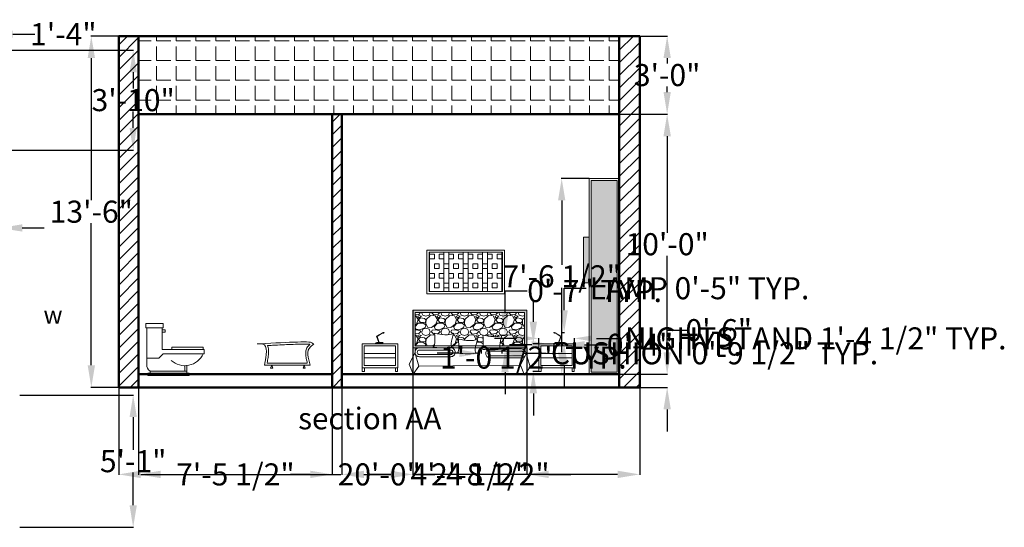
# Model space of a CAD drawing. Units: inches. Extents: x 4451 to 5261, y 886 to 1442.
# Tile 3 of 4: x 4807 to 5261, y 928 to 1162. Entities that reach past the tile are written whole.
import ezdxf

# ---------------------------------------------------------------- set-up
doc = ezdxf.new("R2010")
doc.units = ezdxf.units.IN
doc.header["$MEASUREMENT"] = 0
for name, color, linetype, lineweight in [('A-ANNO-DIMS', 2, 'Continuous', 18), ('A-ANNO-TEXT', 7, 'Continuous', 25), ('A-FLOR-FIXT', 9, 'Continuous', 20), ('A-FURN', 8, 'Continuous', 18), ('A-FURN-PATT', 8, 'Continuous', 13), ('A-SECT', 7, 'Continuous', 50)]:
    doc.layers.add(name, color=color, linetype=linetype, lineweight=lineweight)
doc.layers.add('A-SECT-PATT', color=241, linetype='Continuous', lineweight=13, true_color=0xf7abae)
doc.styles.get("Standard").update_dxf_attribs({"font": 'arial.ttf'})
doc.dimstyles.get("Standard").update_dxf_attribs({"dimtxt": 10.18, "dimasz": 10.18, "dimexe": 0.18, "dimexo": 0.0625, "dimgap": 0.09, "dimtad": 0, "dimtih": 1, "dimtoh": 1, "dimdec": 0, "dimzin": 0, "dimdsep": 46, "dimlunit": 3, "dimtxsty": 'Standard', "dimcen": 0.09, "dimadec": 0, "dimazin": 0, "dimtfac": 1, "dimtdec": 0, "dimtofl": 0, "dimtmove": 0, "dimatfit": 3, "dimfxl": 1, "dimtolj": 1, "dimtzin": 0, "dimarcsym": 0})
pattern_1 = [(45, (-229.911, 0), (-2.9168155, 2.9168155), [])]

# ---------------------------------------------------------------- blocks, each defined once
blk = doc.blocks.new('*U10')
for p, q in [((-0.5, 5), (-0.5, 22)), ((6.5, 22), (6.5, 12)), ((6.5, 21), (8, 21)), ((8, 20), (6.5, 20)), ((8, 21), (8, 20)), ((7, 10), (5, 8)), ((6.5, 12), (26, 12)), ((26, 10), (7, 10)), ((11, 13), (11, 12)), ((25.5, 13), (11, 13)), ((25.5, 12), (25.5, 13)), ((26, 12), (26, 10)), ((5, 8), (-0.5, 8)), ((1, 2), (1, 1)), ((18, 2), (1, 2)), ((17, 4.5), (17, 2)), ((18, 2), (18, 4.5376)), ((18, 1), (18, 2))]:
    blk.add_line(p, q)
for points in [[(-1, 22), (-1, 24), (7, 24), (7, 22)], [(0, 0), (0, 1), (19, 1), (19, 0)]]:
    blk.add_lwpolyline(points, close=True)
for centre, radius, start, end in [((17, 13.7955), 9.3089, 227.7453, 335.9381), ((2.75, 4.75), 3.2596, 175.6013, 237.5288)]:
    blk.add_arc(centre, radius, start, end)
blk = doc.blocks.new('CUSHION-ELEV')
for points in [[(0.79, 6.75), (0.98, 3.53), (1.17, 0.31), (0, 0.27)], [(0.79, 6.75), (4.1, 6.13), (7.4, 5.52), (9.55, 6.75)], [(0, 0.27), (2.47, 0.04), (4.94, -0.18), (9.29, 0.22)]]:
    blk.add_open_spline(points, degree=3)
blk.add_open_spline([(9.55, 6.75), (8.66, 3.34), (7.77, -0.07), (9.51, 0.25), (9.51, 0.25)], degree=3, knots=[0, 0, 0, 0, 6.500705, 6.513641, 6.513641, 6.513641, 6.513641])
blk = doc.blocks.new('NIGHTSTAND-ELEV')
for p, q in [((1, 8.22), (15.46, 8.22)), ((1, 8.22), (15.46, 8.22)), ((1, 6.22), (15.46, 6.22))]:
    blk.add_line(p, q)
for points in [[(0, 12.74), (0, 12.74), (16.46, 12.74), (16.46, 12.74), (16.46, 1.69), (16.46, 1.69), (0, 1.69), (0, 1.69)], [(1, 11.74), (15.46, 11.74), (15.46, 2.69), (1, 2.69)], [(1.07, 1.69), (1.07, 1.69), (0.06, 1.69), (0.06, 1.69), (0.06, 0), (0.06, 0), (1.07, 0), (1.07, 0)], [(16.41, 1.69), (16.41, 1.69), (15.4, 1.69), (15.4, 1.69), (15.4, 0), (15.4, 0), (16.41, 0), (16.41, 0)]]:
    blk.add_lwpolyline(points, close=True)
blk = doc.blocks.new('BEDSIDE-LAMP-ELEV')
for p, q in [((0.39, 4.98), (0, 4.98)), ((3.41, 3.22), (0.39, 4.98)), ((3.22, 3.15), (0.65, 4.7)), ((0.75, 0.34), (0.36, 0)), ((0.36, 0), (4.03, 0)), ((3.35, 0.34), (0.75, 0.34)), ((2.21, 0.34), (3.22, 3.15)), ((2.36, 0.34), (3.41, 3.22)), ((4.03, 0), (3.35, 0.34))]:
    blk.add_line(p, q)
blk.add_arc((0.39, 4.98), 0.387, 180, 329.7191)
blk = doc.blocks.new('*D30')
at = {"layer": 'A-ANNO-DIMS', "color": 0, "lineweight": -2, "transparency": 16777216}
for p, q in [((4777.87, 1159.67), (4777.87, 1155.48)), ((4793.72, 1159.67), (4793.72, 1155.48)), ((4767.69, 1155.66), (4757.51, 1155.66)), ((4803.9, 1155.66), (4814.08, 1155.66))]:
    blk.add_line(p, q, dxfattribs=at)
at = {"layer": 'A-ANNO-DIMS', "color": 0, "transparency": 16777216}
for points in [[(4767.69, 1157.36), (4767.69, 1153.97), (4777.87, 1155.66)], [(4803.9, 1157.36), (4803.9, 1153.97), (4793.72, 1155.66)]]:
    blk.add_solid(points, dxfattribs=at)
at = {"layer": 'Defpoints', "color": 0, "transparency": 16777216}
for p in [(4777.87, 1159.74), (4793.72, 1159.74), (4793.72, 1155.66)]:
    blk.add_point(p, dxfattribs=at)
at = {"layer": 'A-ANNO-DIMS', "color": 0, "transparency": 16777216, "insert": (4827.22, 1155.66), "char_height": 10.18, "attachment_point": 5}
blk.add_mtext('\\A1;1\'-4"', dxfattribs=at)
blk = doc.blocks.new('*D35')
at = {"layer": 'A-ANNO-DIMS', "color": 0, "lineweight": -2, "transparency": 16777216}
for p, q in [((5009.76, 1008.51), (4999.58, 1008.51)), ((5019.94, 1009.88), (5019.94, 1008.33)), ((5029.48, 1009.88), (5029.48, 1008.33)), ((5039.66, 1008.51), (5049.84, 1008.51))]:
    blk.add_line(p, q, dxfattribs=at)
at = {"layer": 'A-ANNO-DIMS', "color": 0, "transparency": 16777216}
for points in [[(5009.76, 1010.2), (5009.76, 1006.81), (5019.94, 1008.51)], [(5039.66, 1010.2), (5039.66, 1006.81), (5029.48, 1008.51)]]:
    blk.add_solid(points, dxfattribs=at)
at = {"layer": 'Defpoints', "color": 0, "transparency": 16777216}
for p in [(5019.94, 1009.94), (5029.48, 1009.94), (5029.48, 1008.51)]:
    blk.add_point(p, dxfattribs=at)
at = {"layer": 'A-ANNO-DIMS', "color": 0, "transparency": 16777216, "insert": (5127.53, 1008.51), "char_height": 10.18, "attachment_point": 5}
blk.add_mtext('\\A1;CUSHION 0\'-9 1/2" TYP.', dxfattribs=at)
blk = doc.blocks.new('*D36')
at = {"layer": 'A-ANNO-DIMS', "color": 0, "lineweight": -2, "transparency": 16777216}
for p, q in [((5030.92, 1027.05), (5030.92, 1037.23)), ((5030.92, 1037.23), (5041.1, 1037.23)), ((5029.55, 1016.87), (5031.1, 1016.87)), ((5029.55, 1009.94), (5031.1, 1009.94)), ((5030.92, 999.76), (5030.92, 989.58))]:
    blk.add_line(p, q, dxfattribs=at)
at = {"layer": 'A-ANNO-DIMS', "color": 0, "transparency": 16777216}
for points in [[(5029.22, 1027.05), (5032.61, 1027.05), (5030.92, 1016.87)], [(5029.22, 999.76), (5032.61, 999.76), (5030.92, 1009.94)]]:
    blk.add_solid(points, dxfattribs=at)
at = {"layer": 'Defpoints', "color": 0, "transparency": 16777216}
for p in [(5029.48, 1016.87), (5030.92, 1016.87), (5029.48, 1009.94)]:
    blk.add_point(p, dxfattribs=at)
at = {"layer": 'A-ANNO-DIMS', "color": 0, "transparency": 16777216, "insert": (5072.21, 1037.23), "char_height": 10.18, "attachment_point": 5}
blk.add_mtext('\\A1;0\'-7" TYP.', dxfattribs=at)
blk = doc.blocks.new('*D37')
at = {"layer": 'A-ANNO-DIMS', "color": 0, "lineweight": -2, "transparency": 16777216}
for p, q in [((5058.17, 1028.33), (5058.17, 1038.51)), ((5058.17, 1038.51), (5068.35, 1038.51)), ((5057.48, 1018.15), (5058.35, 1018.15)), ((5057.48, 1013.17), (5058.35, 1013.17)), ((5058.17, 1002.99), (5058.17, 992.81))]:
    blk.add_line(p, q, dxfattribs=at)
at = {"layer": 'A-ANNO-DIMS', "color": 0, "transparency": 16777216}
for points in [[(5056.47, 1028.33), (5059.86, 1028.33), (5058.17, 1018.15)], [(5056.47, 1002.99), (5059.86, 1002.99), (5058.17, 1013.17)]]:
    blk.add_solid(points, dxfattribs=at)
at = {"layer": 'Defpoints', "color": 0, "transparency": 16777216}
for p in [(5057.42, 1018.15), (5058.17, 1018.15), (5057.42, 1013.17)]:
    blk.add_point(p, dxfattribs=at)
at = {"layer": 'A-ANNO-DIMS', "color": 0, "transparency": 16777216, "insert": (5120.58, 1038.51), "char_height": 10.18, "attachment_point": 5}
blk.add_mtext('\\A1;LAMP 0\'-5" TYP.', dxfattribs=at)
blk = doc.blocks.new('*D38')
at = {"layer": 'A-ANNO-DIMS', "color": 0, "lineweight": -2, "transparency": 16777216}
for p, q in [((5053.39, 1013.1), (5053.39, 1012.24)), ((5057.42, 1013.1), (5057.42, 1012.24)), ((5043.21, 1012.42), (5033.03, 1012.42)), ((5067.6, 1012.42), (5077.78, 1012.42))]:
    blk.add_line(p, q, dxfattribs=at)
at = {"layer": 'A-ANNO-DIMS', "color": 0, "transparency": 16777216}
for points in [[(5043.21, 1014.12), (5043.21, 1010.72), (5053.39, 1012.42)], [(5067.6, 1014.12), (5067.6, 1010.72), (5057.42, 1012.42)]]:
    blk.add_solid(points, dxfattribs=at)
at = {"layer": 'Defpoints', "color": 0, "transparency": 16777216}
for p in [(5053.39, 1013.17), (5057.42, 1013.17), (5057.42, 1012.42)]:
    blk.add_point(p, dxfattribs=at)
at = {"layer": 'A-ANNO-DIMS', "color": 0, "transparency": 16777216, "insert": (5108.9, 1012.42), "char_height": 10.18, "attachment_point": 5}
blk.add_mtext('\\A1;0\'-4" TYP.', dxfattribs=at)
blk = doc.blocks.new('*D39')
at = {"layer": 'A-ANNO-DIMS', "color": 0, "lineweight": -2, "transparency": 16777216}
for p, q in [((5036.25, 1015.37), (5026.07, 1015.37)), ((5046.43, 1012.96), (5046.43, 1015.55)), ((5062.9, 1012.96), (5062.9, 1015.55)), ((5073.08, 1015.37), (5083.26, 1015.37))]:
    blk.add_line(p, q, dxfattribs=at)
at = {"layer": 'A-ANNO-DIMS', "color": 0, "transparency": 16777216}
for points in [[(5036.25, 1017.06), (5036.25, 1013.67), (5046.43, 1015.37)], [(5073.08, 1017.06), (5073.08, 1013.67), (5062.9, 1015.37)]]:
    blk.add_solid(points, dxfattribs=at)
at = {"layer": 'Defpoints', "color": 0, "transparency": 16777216}
for p in [(5046.43, 1012.9), (5062.9, 1015.37), (5062.9, 1012.9)]:
    blk.add_point(p, dxfattribs=at)
at = {"layer": 'A-ANNO-DIMS', "color": 0, "transparency": 16777216, "insert": (5174.18, 1015.37), "char_height": 10.18, "attachment_point": 5}
blk.add_mtext('\\A1;NIGHTSTAND 1\'-4 1/2" TYP.', dxfattribs=at)
blk = doc.blocks.new('*D40')
at = {"layer": 'A-ANNO-DIMS', "color": 0, "lineweight": -2, "transparency": 16777216}
for p, q in [((5043.96, 1023.08), (5043.96, 1033.26)), ((5046.37, 1012.9), (5043.78, 1012.9)), ((5046.37, 1000.16), (5043.78, 1000.16)), ((5043.96, 989.98), (5043.96, 979.8))]:
    blk.add_line(p, q, dxfattribs=at)
at = {"layer": 'A-ANNO-DIMS', "color": 0, "transparency": 16777216}
for points in [[(5042.27, 1023.08), (5045.66, 1023.08), (5043.96, 1012.9)], [(5042.27, 989.98), (5045.66, 989.98), (5043.96, 1000.16)]]:
    blk.add_solid(points, dxfattribs=at)
at = {"layer": 'Defpoints', "color": 0, "transparency": 16777216}
for p in [(5043.96, 1012.9), (5046.43, 1012.9), (5046.43, 1000.16)]:
    blk.add_point(p, dxfattribs=at)
at = {"layer": 'A-ANNO-DIMS', "color": 0, "transparency": 16777216, "insert": (5043.96, 1006.53), "char_height": 10.18, "attachment_point": 5}
blk.add_mtext('\\A1;1\'-0 1/2" TYP.', dxfattribs=at)
blk = doc.blocks.new('*D44')
at = {"layer": 'A-ANNO-DIMS', "color": 0, "lineweight": -2, "transparency": 16777216}
for p, q in [((4807.16, 989.25), (4859.61, 989.25)), ((4859.43, 979.07), (4859.43, 964.04)), ((4859.43, 938.43), (4859.43, 953.46)), ((4807.16, 928.25), (4859.61, 928.25))]:
    blk.add_line(p, q, dxfattribs=at)
at = {"layer": 'A-ANNO-DIMS', "color": 0, "transparency": 16777216}
for points in [[(4857.74, 979.07), (4861.13, 979.07), (4859.43, 989.25)], [(4857.74, 938.43), (4861.13, 938.43), (4859.43, 928.25)]]:
    blk.add_solid(points, dxfattribs=at)
at = {"layer": 'Defpoints', "color": 0, "transparency": 16777216}
for p in [(4807.09, 989.25), (4859.43, 989.25), (4807.09, 928.25)]:
    blk.add_point(p, dxfattribs=at)
at = {"layer": 'A-ANNO-DIMS', "color": 0, "transparency": 16777216, "insert": (4859.43, 958.75), "char_height": 10.18, "attachment_point": 5}
blk.add_mtext('\\A1;5\'-1"', dxfattribs=at)
blk = doc.blocks.new('*D45')
at = {"layer": 'A-ANNO-DIMS', "color": 0, "lineweight": -2, "transparency": 16777216}
for p, q in [((4798.16, 1148.25), (4859.61, 1148.25)), ((4859.43, 1138.07), (4859.43, 1130.54)), ((4859.43, 1112.43), (4859.43, 1119.96)), ((4798.16, 1102.25), (4859.61, 1102.25))]:
    blk.add_line(p, q, dxfattribs=at)
at = {"layer": 'A-ANNO-DIMS', "color": 0, "transparency": 16777216}
for points in [[(4857.74, 1138.07), (4861.13, 1138.07), (4859.43, 1148.25)], [(4857.74, 1112.43), (4861.13, 1112.43), (4859.43, 1102.25)]]:
    blk.add_solid(points, dxfattribs=at)
at = {"layer": 'Defpoints', "color": 0, "transparency": 16777216}
for p in [(4798.09, 1148.25), (4859.43, 1148.25), (4798.09, 1102.25)]:
    blk.add_point(p, dxfattribs=at)
at = {"layer": 'A-ANNO-DIMS', "color": 0, "transparency": 16777216, "insert": (4859.43, 1125.25), "char_height": 10.18, "attachment_point": 5}
blk.add_mtext('\\A1;3\'-10"', dxfattribs=at)
blk = doc.blocks.new('*D55')
at = {"layer": 'A-ANNO-DIMS', "color": 0, "lineweight": -2, "transparency": 16777216}
for p, q in [((4786.59, 1093.19), (4786.59, 1066.12)), ((4798.09, 1093.19), (4798.09, 1066.12)), ((4776.41, 1066.3), (4766.23, 1066.3)), ((4808.27, 1066.3), (4818.45, 1066.3))]:
    blk.add_line(p, q, dxfattribs=at)
at = {"layer": 'A-ANNO-DIMS', "color": 0, "transparency": 16777216}
for points in [[(4776.41, 1068), (4776.41, 1064.61), (4786.59, 1066.3)], [(4808.27, 1068), (4808.27, 1064.61), (4798.09, 1066.3)]]:
    blk.add_solid(points, dxfattribs=at)
at = {"layer": 'Defpoints', "color": 0, "transparency": 16777216}
for p in [(4786.59, 1093.25), (4798.09, 1093.25), (4786.59, 1066.3)]:
    blk.add_point(p, dxfattribs=at)
at = {"layer": 'A-ANNO-DIMS', "color": 0, "transparency": 16777216, "insert": (4736.8, 1066.3), "char_height": 10.18, "attachment_point": 5}
blk.add_mtext('\\A1;0\'-11 1/2"', dxfattribs=at)
blk = doc.blocks.new('*D72')
at = {"layer": 'A-ANNO-DIMS', "color": 0, "lineweight": -2, "transparency": 16777216}
for p, q in [((4852.77, 992.74), (4852.77, 952.47)), ((5093.02, 992.74), (5093.02, 952.47)), ((4862.95, 952.65), (4955.24, 952.65)), ((5082.84, 952.65), (4990.56, 952.65))]:
    blk.add_line(p, q, dxfattribs=at)
at = {"layer": 'A-ANNO-DIMS', "color": 0, "transparency": 16777216}
for points in [[(4862.95, 954.35), (4862.95, 950.96), (4852.77, 952.65)], [(5082.84, 954.35), (5082.84, 950.96), (5093.02, 952.65)]]:
    blk.add_solid(points, dxfattribs=at)
at = {"layer": 'Defpoints', "color": 0, "transparency": 16777216}
for p in [(4852.77, 992.8), (5093.02, 992.8), (5093.02, 952.65)]:
    blk.add_point(p, dxfattribs=at)
at = {"layer": 'A-ANNO-DIMS', "color": 0, "transparency": 16777216, "insert": (4972.9, 952.65), "char_height": 10.18, "attachment_point": 5}
blk.add_mtext('\\A1;20\'-0"', dxfattribs=at)
blk = doc.blocks.new('*D73')
at = {"layer": 'A-ANNO-DIMS', "color": 0, "lineweight": -2, "transparency": 16777216}
for p, q in [((4852.71, 1154.8), (4839.94, 1154.8)), ((4840.12, 1144.62), (4840.12, 1079.09)), ((4840.12, 1002.98), (4840.12, 1068.51)), ((4852.71, 992.8), (4839.94, 992.8))]:
    blk.add_line(p, q, dxfattribs=at)
at = {"layer": 'A-ANNO-DIMS', "color": 0, "transparency": 16777216}
for points in [[(4838.43, 1144.62), (4841.82, 1144.62), (4840.12, 1154.8)], [(4838.43, 1002.98), (4841.82, 1002.98), (4840.12, 992.8)]]:
    blk.add_solid(points, dxfattribs=at)
at = {"layer": 'Defpoints', "color": 0, "transparency": 16777216}
for p in [(4840.12, 1154.8), (4852.77, 1154.8), (4852.77, 992.8)]:
    blk.add_point(p, dxfattribs=at)
at = {"layer": 'A-ANNO-DIMS', "color": 0, "transparency": 16777216, "insert": (4840.12, 1073.8), "char_height": 10.18, "attachment_point": 5}
blk.add_mtext('\\A1;13\'-6"', dxfattribs=at)
blk = doc.blocks.new('*D74')
at = {"layer": 'A-ANNO-DIMS', "color": 0, "lineweight": -2, "transparency": 16777216}
for p, q in [((5083.66, 1118.8), (5105.85, 1118.8)), ((5105.67, 1108.62), (5105.67, 1064.09)), ((5105.67, 1008.98), (5105.67, 1053.51)), ((5083.66, 998.8), (5105.85, 998.8))]:
    blk.add_line(p, q, dxfattribs=at)
at = {"layer": 'A-ANNO-DIMS', "color": 0, "transparency": 16777216}
for points in [[(5103.98, 1108.62), (5107.37, 1108.62), (5105.67, 1118.8)], [(5103.98, 1008.98), (5107.37, 1008.98), (5105.67, 998.8)]]:
    blk.add_solid(points, dxfattribs=at)
at = {"layer": 'Defpoints', "color": 0, "transparency": 16777216}
for p in [(5083.6, 1118.8), (5105.67, 1118.8), (5083.6, 998.8)]:
    blk.add_point(p, dxfattribs=at)
at = {"layer": 'A-ANNO-DIMS', "color": 0, "transparency": 16777216, "insert": (5105.67, 1058.8), "char_height": 10.18, "attachment_point": 5}
blk.add_mtext('\\A1;10\'-0"', dxfattribs=at)
blk = doc.blocks.new('*D75')
at = {"layer": 'A-ANNO-DIMS', "color": 0, "lineweight": -2, "transparency": 16777216}
for p, q in [((4861.87, 998.74), (4861.87, 952.47)), ((4951.24, 998.74), (4951.24, 952.47)), ((4872.05, 952.65), (4881.12, 952.65)), ((4941.06, 952.65), (4932, 952.65))]:
    blk.add_line(p, q, dxfattribs=at)
at = {"layer": 'A-ANNO-DIMS', "color": 0, "transparency": 16777216}
for points in [[(4872.05, 954.35), (4872.05, 950.96), (4861.87, 952.65)], [(4941.06, 954.35), (4941.06, 950.96), (4951.24, 952.65)]]:
    blk.add_solid(points, dxfattribs=at)
at = {"layer": 'Defpoints', "color": 0, "transparency": 16777216}
for p in [(4861.87, 998.8), (4951.24, 998.8), (4951.24, 952.65)]:
    blk.add_point(p, dxfattribs=at)
at = {"layer": 'A-ANNO-DIMS', "color": 0, "transparency": 16777216, "insert": (4906.56, 952.65), "char_height": 10.18, "attachment_point": 5}
blk.add_mtext('\\A1;7\'-5 1/2"', dxfattribs=at)
blk = doc.blocks.new('*D76')
at = {"layer": 'A-ANNO-DIMS', "color": 0, "lineweight": -2, "transparency": 16777216}
for p, q in [((5105.67, 1008.98), (5105.67, 1019.16)), ((5105.67, 1019.16), (5115.85, 1019.16)), ((5083.66, 998.8), (5105.85, 998.8)), ((5083.66, 992.8), (5105.85, 992.8)), ((5105.67, 982.62), (5105.67, 972.44))]:
    blk.add_line(p, q, dxfattribs=at)
at = {"layer": 'A-ANNO-DIMS', "color": 0, "transparency": 16777216}
for points in [[(5103.98, 1008.98), (5107.37, 1008.98), (5105.67, 998.8)], [(5103.98, 982.62), (5107.37, 982.62), (5105.67, 992.8)]]:
    blk.add_solid(points, dxfattribs=at)
at = {"layer": 'Defpoints', "color": 0, "transparency": 16777216}
for p in [(5083.6, 998.8), (5105.67, 998.8), (5083.6, 992.8)]:
    blk.add_point(p, dxfattribs=at)
at = {"layer": 'A-ANNO-DIMS', "color": 0, "transparency": 16777216, "insert": (5129.47, 1019.16), "char_height": 10.18, "attachment_point": 5}
blk.add_mtext('\\A1;0\'-6"', dxfattribs=at)
blk = doc.blocks.new('*D77')
at = {"layer": 'A-ANNO-DIMS', "color": 0, "lineweight": -2, "transparency": 16777216}
for p, q in [((5083.66, 1154.8), (5105.85, 1154.8)), ((5105.67, 1144.62), (5105.67, 1142.09)), ((5105.67, 1128.98), (5105.67, 1131.51)), ((5083.66, 1118.8), (5105.85, 1118.8))]:
    blk.add_line(p, q, dxfattribs=at)
at = {"layer": 'A-ANNO-DIMS', "color": 0, "transparency": 16777216}
for points in [[(5103.98, 1144.62), (5107.37, 1144.62), (5105.67, 1154.8)], [(5103.98, 1128.98), (5107.37, 1128.98), (5105.67, 1118.8)]]:
    blk.add_solid(points, dxfattribs=at)
at = {"layer": 'Defpoints', "color": 0, "transparency": 16777216}
for p in [(5083.6, 1154.8), (5105.67, 1154.8), (5083.6, 1118.8)]:
    blk.add_point(p, dxfattribs=at)
at = {"layer": 'A-ANNO-DIMS', "color": 0, "transparency": 16777216, "insert": (5105.67, 1136.8), "char_height": 10.18, "attachment_point": 5}
blk.add_mtext('\\A1;3\'-0"', dxfattribs=at)
blk = doc.blocks.new('*D78')
at = {"layer": 'A-ANNO-DIMS', "color": 0, "lineweight": -2, "transparency": 16777216}
for p, q in [((4988.39, 1028.26), (4988.39, 952.47)), ((4955.66, 998.74), (4955.66, 952.47)), ((4965.84, 952.65), (4978.21, 952.65)), ((4988.39, 952.65), (4998.57, 952.65))]:
    blk.add_line(p, q, dxfattribs=at)
at = {"layer": 'A-ANNO-DIMS', "color": 0, "transparency": 16777216}
for points in [[(4965.84, 954.35), (4965.84, 950.96), (4955.66, 952.65)], [(4978.21, 954.35), (4978.21, 950.96), (4988.39, 952.65)]]:
    blk.add_solid(points, dxfattribs=at)
at = {"layer": 'Defpoints', "color": 0, "transparency": 16777216}
for p in [(4988.39, 1028.32), (4955.66, 998.8), (4988.39, 952.65)]:
    blk.add_point(p, dxfattribs=at)
at = {"layer": 'A-ANNO-DIMS', "color": 0, "transparency": 16777216, "insert": (5024.14, 952.65), "char_height": 10.18, "attachment_point": 5}
blk.add_mtext('\\A1;2\'-8 1/2"', dxfattribs=at)
blk = doc.blocks.new('*D79')
at = {"layer": 'A-ANNO-DIMS', "color": 0, "lineweight": -2, "transparency": 16777216}
for p, q in [((4988.39, 1010.95), (4988.39, 952.47)), ((5040.92, 1010.95), (5040.92, 952.47)), ((4978.21, 952.65), (4968.03, 952.65)), ((5051.1, 952.65), (5061.28, 952.65))]:
    blk.add_line(p, q, dxfattribs=at)
at = {"layer": 'A-ANNO-DIMS', "color": 0, "transparency": 16777216}
for points in [[(4978.21, 954.35), (4978.21, 950.96), (4988.39, 952.65)], [(5051.1, 954.35), (5051.1, 950.96), (5040.92, 952.65)]]:
    blk.add_solid(points, dxfattribs=at)
at = {"layer": 'Defpoints', "color": 0, "transparency": 16777216}
for p in [(4988.39, 1011.01), (5040.92, 1011.01), (5040.92, 952.65)]:
    blk.add_point(p, dxfattribs=at)
at = {"layer": 'A-ANNO-DIMS', "color": 0, "transparency": 16777216, "insert": (5014.65, 952.65), "char_height": 10.18, "attachment_point": 5}
blk.add_mtext('\\A1;4\'-4 1/2"', dxfattribs=at)
blk = doc.blocks.new('*D80')
at = {"layer": 'A-ANNO-DIMS', "color": 0, "lineweight": -2, "transparency": 16777216}
for p, q in [((5069.63, 1089.17), (5056.86, 1089.17)), ((5057.04, 1078.99), (5057.04, 1049.34)), ((5057.04, 1008.98), (5057.04, 1038.63)), ((5069.63, 998.8), (5056.86, 998.8))]:
    blk.add_line(p, q, dxfattribs=at)
at = {"layer": 'A-ANNO-DIMS', "color": 0, "transparency": 16777216}
for points in [[(5055.34, 1078.99), (5058.73, 1078.99), (5057.04, 1089.17)], [(5055.34, 1008.98), (5058.73, 1008.98), (5057.04, 998.8)]]:
    blk.add_solid(points, dxfattribs=at)
at = {"layer": 'Defpoints', "color": 0, "transparency": 16777216}
for p in [(5057.04, 1089.17), (5069.69, 1089.17), (5069.69, 998.8)]:
    blk.add_point(p, dxfattribs=at)
at = {"layer": 'A-ANNO-DIMS', "color": 0, "transparency": 16777216, "insert": (5057.04, 1043.98), "char_height": 10.18, "attachment_point": 5}
blk.add_mtext('\\A1;7\'-6 1/2"', dxfattribs=at)

msp = doc.modelspace()

# ---------------------------------------------------------------- hatches: boundary and pattern name
at = {"layer": 'A-FURN-PATT'}
h = msp.add_hatch(color=256, dxfattribs=at)
h.dxf.hatch_style = 1
h.paths.add_polyline_path([(5070.69, 999.8), (5082.6, 999.8), (5082.6, 1088.17), (5070.69, 1088.17)])
h = msp.add_hatch(color=256, dxfattribs=at)
h.dxf.hatch_style = 1
h.paths.add_polyline_path([(5069.69, 1062.01), (5067.12, 1062.01), (5067.12, 1040.97), (5069.69, 1040.97)])
h = msp.add_hatch(dxfattribs=at)
h.set_pattern_fill('BOX', color=256, scale=8.9)
h.set_pattern_definition([(90, (-248.247, -51.5795), (-8.9, 5e-16), []), (90, (-246.022, -51.5795), (-8.9, 5e-16), []), (0, (-248.247, -51.5795), (0, 8.9), [-2.225, 2.225]), (0, (-248.247, -49.3545), (0, 8.9), [-2.225, 2.225]), (0, (-248.247, -47.1295), (0, 8.9), [2.225, -2.225]), (0, (-248.247, -44.9045), (0, 8.9), [2.225, -2.225]), (90, (-243.797, -51.5795), (-8.9, 5e-16), [2.225, -2.225]), (90, (-241.572, -51.5795), (-8.9, 5e-16), [2.225, -2.225])])
h.paths.add_polyline_path([(5029.68, 1036.95), (5029.68, 1055.09), (4995.86, 1055.09), (4995.86, 1036.95)])
h = msp.add_hatch(color=256, dxfattribs=at)
h.dxf.hatch_style = 1
edge = h.paths.add_edge_path()
edge.add_line((4988.39, 1028.32), (4988.39, 1011.01))
edge.add_line((4988.39, 1011.01), (5002.61, 1011.01))
edge.add_spline(control_points=[(5002.61, 1011.01), (5000.64, 1011), (4999.12, 1011.14), (4997.6, 1011.28)], knot_values=[0, 0, 0, 0, 5.728069, 5.728069, 5.728069, 5.728069], degree=3, periodic=0)
edge.add_spline(control_points=[(4997.6, 1011.28), (4997.93, 1011.29), (4998.15, 1011.56), (4998.29, 1012.01)], knot_values=[4.269883, 4.269883, 4.269883, 4.269883, 5.96329, 5.96329, 5.96329, 5.96329], degree=3, periodic=0)
edge.add_line((4998.29, 1012.01), (4989.39, 1012.01))
edge.add_line((4989.39, 1012.01), (4989.39, 1027.32))
edge.add_line((4989.39, 1027.32), (5039.92, 1027.32))
edge.add_line((5039.92, 1027.32), (5039.92, 1012.01))
edge.add_line((5039.92, 1012.01), (5028.46, 1012.01))
edge.add_spline(control_points=[(5028.46, 1012.01), (5028.44, 1011.61), (5028.45, 1011.28), (5028.51, 1011.01)], knot_values=[3.442208, 3.442208, 3.442208, 3.442208, 4.5249, 4.5249, 4.5249, 4.5249], degree=3, periodic=0)
edge.add_line((5028.51, 1011.01), (5040.92, 1011.01))
edge.add_line((5040.92, 1011.01), (5040.92, 1028.32))
edge.add_line((5040.92, 1028.32), (4988.39, 1028.32))
h = msp.add_hatch(dxfattribs=at)
h.set_pattern_fill('GRAVEL', color=256, scale=8.9)
h.set_pattern_definition([(228.012788, (-223.5031, 3.7945), (-71.2, -80.1), [1.19737, -118.539884]), (184.969741, (-224.3041, 2.90448), (106.8, 8.9), [2.054725, -203.41773]), (132.510447, (-226.3511, 2.7265), (89, -97.9), [1.448813, -143.43269]), (267.273689, (-229.8221, 0.50148), (8.9, 178), [1.871118, -185.240667]), (292.833654, (-229.9111, -1.36752), (-44.5, 106.8), [1.83478, -181.643421]), (357.273689, (-229.1991, -3.05852), (-178, 8.9), [1.871118, -185.240667]), (37.6942405, (-227.3301, -3.14752), (-115.7, -89), [2.474458, -244.971152]), (72.2553284, (-225.3721, -1.63452), (62.3, 195.8), [2.336143, -231.278261]), (121.429566, (-224.6601, 0.59048), (-71.2, 115.7), [1.877455, -185.86825]), (175.236358, (-225.6391, 2.1925), (97.9, -8.9), [2.143405, -105.026787]), (222.397438, (-227.7751, 2.37048), (-106.8, -97.9), [2.771887, -274.417038]), (138.814075, (-221.0111, 0.4125), (-62.3, 53.4), [0.946079, -93.662219]), (171.469234, (-221.7231, 1.03548), (115.7, -17.8), [1.79991, -178.191452]), (225, (-223.503, 1.3025), (-1e-15, -8.9), [1.258647, -11.327854]), (203.19859, (-224.1261, 2.3705), (44.5, 17.8), [0.677806, -67.102574]), (291.80141, (-224.7491, 2.1035), (-8.9, 26.7), [0.958557, -46.96941]), (30.963757, (-224.3931, 1.2135), (26.7, 17.8), [1.556868, -50.338604]), (161.56505, (-223.058, 2.0145), (17.8, -8.9), [1.12577, -27.018501]), (16.38954, (-229.9111, 2.1035), (89, 26.7), [1.57708, -156.131322]), (70.346176, (-228.3981, 2.5485), (-35.6, -97.9), [1.323083, -130.984929]), (293.19859, (-223.0581, 3.7945), (-17.8, 44.5), [1.355603, -66.424777]), (343.61046, (-222.5241, 2.5485), (-89, 26.7), [1.57708, -156.131322]), (339.443955, (-229.9111, -3.4145), (-44.5, 17.8), [1.520832, -74.520801]), (294.77514, (-228.4871, -3.9485), (-44.5, 97.9), [1.274284, -126.154323]), (66.80141, (-222.9691, -5.1055), (17.8, 44.5), [1.355603, -66.424777]), (17.354025, (-222.4351, -3.8595), (-115.7, -35.6), [1.491916, -147.69927]), (69.443955, (-227.3301, -5.1055), (-17.8, -44.5), [0.760416, -75.281217]), (101.309932, (-223.5031, -5.1055), (-8.9, 35.6), [0.453811, -44.927463]), (165.963757, (-223.592, -4.6605), (26.7, -8.9), [1.83478, -34.86086]), (186.009006, (-225.3721, -4.21552), (89, 8.9), [1.700345, -168.333916]), (303.69007, (-224.393, 0.4125), (-8.9, 17.8), [1.283576, -30.80583]), (353.1572266, (-223.6811, -0.65552), (151.3, -17.8), [2.240967, -221.855307]), (60.945396, (-221.4561, -0.9225), (-35.6, -62.3), [0.916308, -90.7148]), (90, (-221.011, -0.1215), (-8.9, 8.9), [0.534, -8.366]), (120.256437, (-225.5501, -3.9485), (35.6, -62.3), [1.236424, -122.406328]), (48.012788, (-226.1731, -2.8805), (71.2, 80.1), [2.394741, -117.342513]), (0, (-224.571, -1.1005), (8.9, 8.9), [2.314, -6.586]), (325.304846, (-222.2571, -1.1005), (89, -62.3), [1.407215, -139.314141]), (254.054604, (-221.1001, -1.9015), (-8.9, -35.6), [1.295858, -63.49712]), (207.645975, (-221.4561, -3.14752), (-169.1, -89), [2.109879, -208.87832]), (175.426079, (-223.3251, -4.12652), (-115.7, 8.9), [2.232111, -220.978753])])
edge = h.paths.add_edge_path()
edge.add_spline(control_points=[(5007.14, 1017.75), (5006.54, 1015.46), (5005.95, 1013.17), (5006.15, 1012.01)], knot_values=[0, 0, 0, 0, 4.377261, 4.377261, 4.377261, 4.377261], degree=3, periodic=0)
edge.add_line((5006.15, 1012.01), (5009.57, 1012.01))
edge.add_spline(control_points=[(5009.57, 1012.01), (5009.56, 1012.95), (5009.5, 1014), (5009.43, 1015.05)], knot_values=[0, 0, 0, 0, 1.947045, 1.947045, 1.947045, 1.947045], degree=3, periodic=0)
edge.add_spline(control_points=[(5009.43, 1015.05), (5012.74, 1014.44), (5016.04, 1013.82), (5018.19, 1015.05)], knot_values=[0, 0, 0, 0, 8.589129, 8.589129, 8.589129, 8.589129], degree=3, periodic=0)
edge.add_spline(control_points=[(5018.19, 1015.05), (5017.91, 1014), (5017.64, 1012.95), (5017.44, 1012.01)], knot_values=[0, 0, 0, 0, 2.004065, 2.004065, 2.004065, 2.004065], degree=3, periodic=0)
edge.add_line((5017.44, 1012.01), (5020.81, 1012.01))
edge.add_spline(control_points=[(5020.81, 1012.01), (5020.94, 1013.25), (5020.84, 1015.06), (5020.73, 1016.87)], knot_values=[0, 0, 0, 0, 3.349293, 3.349293, 3.349293, 3.349293], degree=3, periodic=0)
edge.add_spline(control_points=[(5020.73, 1016.87), (5024.03, 1016.25), (5027.34, 1015.64), (5029.48, 1016.87)], knot_values=[0, 0, 0, 0, 8.589129, 8.589129, 8.589129, 8.589129], degree=3, periodic=0)
edge.add_spline(control_points=[(5029.48, 1016.87), (5029.01, 1015.06), (5028.54, 1013.26), (5028.46, 1012.01)], knot_values=[0, 0, 0, 0, 3.442208, 3.442208, 3.442208, 3.442208], degree=3, periodic=0)
edge.add_line((5028.46, 1012.01), (5039.92, 1012.01))
edge.add_line((5039.92, 1012.01), (5039.92, 1027.32))
edge.add_line((5039.92, 1027.32), (4989.39, 1027.32))
edge.add_line((4989.39, 1027.32), (4989.39, 1012.01))
edge.add_line((4989.39, 1012.01), (4998.29, 1012.01))
edge.add_spline(control_points=[(4998.29, 1012.01), (4998.66, 1013.15), (4998.52, 1015.45), (4998.39, 1017.75)], knot_values=[0, 0, 0, 0, 4.269883, 4.269883, 4.269883, 4.269883], degree=3, periodic=0)
edge.add_spline(control_points=[(4998.39, 1017.75), (5001.69, 1017.14), (5004.99, 1016.53), (5007.14, 1017.75)], knot_values=[0, 0, 0, 0, 8.589129, 8.589129, 8.589129, 8.589129], degree=3, periodic=0)
at = {"layer": 'A-SECT-PATT'}
h = msp.add_hatch(dxfattribs=at)
h.set_pattern_fill('ANSI31', color=256, scale=33)
h.set_pattern_definition(pattern_1)
h.paths.add_polyline_path([(4852.77, 992.8), (4861.87, 992.8), (4861.87, 1154.8), (4852.77, 1154.8)])
h.paths.add_polyline_path([(5093.02, 1154.8), (5083.6, 1154.8), (5083.6, 992.8), (5093.02, 992.8)])
h = msp.add_hatch(dxfattribs=at)
h.set_pattern_fill('ANGLE', color=256, scale=33)
h.set_pattern_definition([(0, (-229.911, 0), (0, 9.075), [6.6, -2.475]), (90, (-229.911, 0), (-9.075, 6e-16), [6.6, -2.475])])
h.paths.add_polyline_path([(4861.87, 1154.8), (4861.87, 1118.8), (5083.6, 1118.8), (5083.6, 1154.8)])
h = msp.add_hatch(dxfattribs=at)
h.set_pattern_fill('ANSI31', color=256, scale=33)
h.set_pattern_definition(pattern_1)
h.paths.add_polyline_path([(4955.66, 1118.8), (4951.24, 1118.8), (4951.24, 992.8), (4955.66, 992.8)])

# ---------------------------------------------------------------- linework, layer by layer
at = {"layer": 'A-FLOR-FIXT'}
for p, q in [((4921.15, 1003.98), (4939.73, 1003.98)), ((4919.92, 1002.98), (4941.03, 1002.98)), ((4923.33, 1002.98), (4922.82, 1001.61)), ((4922.82, 1001.61), (4923.85, 1001.61)), ((4923.85, 1001.61), (4923.33, 1002.98)), ((4938.26, 1002.98), (4937.76, 1001.61)), ((4937.76, 1001.61), (4938.78, 1001.61)), ((4938.78, 1001.61), (4938.26, 1002.98))]:
    msp.add_line(p, q, dxfattribs=at)
for points, knots in [([(4919.92, 1002.98), (4920.87, 1007.56), (4922.04, 1013.28), (4917.57, 1012.87), (4916.68, 1012.79)], [0, 0, 0, 0, 9.844777, 12.289625, 12.289625, 12.289625, 12.289625]), ([(4921.42, 1012.06), (4922.19, 1012.1), (4922.95, 1012.14), (4926.72, 1012.34), (4929.59, 1012.49), (4933.65, 1012.65), (4935.06, 1012.69), (4937.3, 1012.73), (4938.2, 1012.74), (4939.56, 1012.72), (4940.08, 1012.7), (4940.67, 1012.66), (4940.83, 1012.64), (4940.96, 1012.62)], [2.659861, 2.659861, 2.659861, 2.659861, 3.979585, 3.979585, 9.285699, 9.285699, 12.483561, 12.483561, 15.077802, 15.077802, 17.144834, 17.144834, 18.044408, 18.044408, 18.044408, 18.044408]), ([(4939.73, 1003.98), (4939.54, 1004.67), (4939.38, 1005.36), (4939.1, 1006.81), (4939, 1007.56), (4938.99, 1008.93), (4939.05, 1009.54), (4939.39, 1010.73), (4939.67, 1011.3), (4940.19, 1011.92), (4940.3, 1012.05), (4940.5, 1012.23), (4940.58, 1012.3), (4940.71, 1012.42), (4940.77, 1012.46), (4940.88, 1012.55), (4940.92, 1012.59), (4940.96, 1012.62)], [1.062845, 1.062845, 1.062845, 1.062845, 2.790616, 2.790616, 4.735848, 4.735848, 6.367727, 6.367727, 7.999606, 7.999606, 8.424348, 8.424348, 8.670353, 8.670353, 8.916358, 8.916358, 9.093128, 9.093128, 9.093128, 9.093128]), ([(4941.03, 1002.98), (4940.11, 1006.34), (4939.18, 1009.71), (4941.19, 1011.51), (4941.25, 1011.56), (4941.32, 1011.62), (4941.39, 1011.68), (4941.85, 1012.06), (4942.31, 1012.44), (4942.77, 1012.83)], [0, 0, 0, 0, 8.529576, 8.529576, 8.529576, 8.803552, 8.803552, 8.803552, 10.66962, 10.66962, 10.66962, 10.66962]), ([(4921.15, 1003.98), (4921.15, 1004.01), (4921.16, 1004.04), (4921.34, 1004.92), (4921.5, 1005.77), (4921.75, 1007.43), (4921.85, 1008.23), (4921.9, 1009.75), (4921.87, 1010.47), (4921.65, 1011.45), (4921.56, 1011.76), (4921.42, 1012.06)], [0.859424, 0.859424, 0.859424, 0.859424, 0.92007, 0.92007, 2.760211, 2.760211, 4.62805, 4.62805, 6.495889, 6.495889, 7.391416, 7.391416, 7.391416, 7.391416]), ([(4921.15, 1003.98), (4921.15, 1004.01), (4921.16, 1004.04), (4921.34, 1004.92), (4921.5, 1005.77), (4921.75, 1007.43), (4921.85, 1008.23), (4921.9, 1009.75), (4921.87, 1010.47), (4921.65, 1011.45), (4921.56, 1011.76), (4921.42, 1012.06)], [0.859424, 0.859424, 0.859424, 0.859424, 0.92007, 0.92007, 2.760211, 2.760211, 4.62805, 4.62805, 6.495889, 6.495889, 7.391416, 7.391416, 7.391416, 7.391416])]:
    msp.add_open_spline(points, degree=3, knots=knots, dxfattribs=at)
for points in [[(4918.31, 1012.88), (4930.82, 1013.59), (4942.8, 1014.22), (4941.95, 1013.19)], [(4919.13, 1012.79), (4919.16, 1012.78), (4919.2, 1012.77), (4919.24, 1012.76)], [(4941.95, 1013.19), (4942.24, 1012.96), (4942.53, 1012.73), (4942.77, 1012.83)]]:
    msp.add_open_spline(points, degree=3, dxfattribs=at)
at = {"layer": 'A-FURN'}
for p, q in [((4988.39, 1028.32), (5040.92, 1028.32)), ((4989.39, 1027.32), (5039.92, 1027.32)), ((5039.92, 1027.32), (5039.92, 1012.01)), ((5040.92, 1028.32), (5040.92, 1011.01)), ((4989.39, 1008.92), (4986.65, 1003.43)), ((4988.39, 1011.01), (5040.92, 1011.01)), ((4989.39, 1012.01), (5039.92, 1012.01)), ((4991.21, 1002.6), (4989.48, 1008.35)), ((5040.67, 1008.4), (5037.99, 1003.01)), ((5042.55, 1002.18), (5040.67, 1008.4)), ((4986.65, 1003.43), (4988.52, 998.8)), ((4988.52, 998.8), (4991.21, 1002.6)), ((4991.21, 1002.6), (5037.99, 1003.01)), ((5037.99, 1003.01), (5039.85, 998.39)), ((5039.85, 998.39), (5042.55, 1002.18)), ((4988.52, 998.8), (5039.68, 998.8))]:
    msp.add_line(p, q, dxfattribs=at)
for points in [[(5083.6, 1089.17), (5083.6, 1089.17), (5069.69, 1089.17), (5069.69, 1089.17), (5069.69, 998.8), (5069.69, 998.8), (5083.6, 998.8), (5083.6, 998.8)], [(5082.6, 1088.17), (5070.69, 1088.17), (5070.69, 999.8), (5082.6, 999.8)], [(5069.69, 1062.01), (5069.69, 1062.01), (5067.12, 1062.01), (5067.12, 1062.01), (5067.12, 1040.97), (5067.12, 1040.97), (5069.69, 1040.97), (5069.69, 1040.97)], [(5069.69, 1062.01), (5069.69, 1062.01), (5069.69, 1062.01), (5069.69, 1062.01), (5069.69, 1051.91), (5069.69, 1051.91), (5069.69, 1051.91), (5069.69, 1051.91)], [(4994.86, 1056.09), (5030.68, 1056.09), (5030.68, 1035.95), (4994.86, 1035.95)], [(4995.86, 1055.09), (4995.86, 1055.09), (5029.68, 1055.09), (5029.68, 1055.09), (5029.68, 1036.95), (5029.68, 1036.95), (4995.86, 1036.95), (4995.86, 1036.95)]]:
    msp.add_lwpolyline(points, close=True, dxfattribs=at)
for points in [[(4988.39, 1011.01), (4988.39, 1028.32), (4988.39, 1028.32), (4988.69, 1028.32), (4988.69, 1028.32)], [(4989.39, 1012.01), (4989.39, 1027.32)], [(4989.39, 1008.92), (4989.39, 1011.01)], [(4988.69, 998.8), (4988.69, 998.8), (4988.39, 998.8), (4988.39, 998.8)]]:
    msp.add_lwpolyline(points, dxfattribs=at)
for points in [[(4989.39, 1009.01, -0.414214), (4991.39, 1011.01), (5005.88, 1011.01, -0.414214), (5007.88, 1009.01), (5007.88, 1008.92, -0.414214), (5005.88, 1006.92), (4991.39, 1006.92, -0.414214), (4989.39, 1008.92)], [(4990.39, 1009.01, -0.414214), (4991.39, 1010.01), (5005.88, 1010.01, -0.414214), (5006.88, 1009.01), (5006.88, 1008.92, -0.414214), (5005.88, 1007.92), (4991.39, 1007.92, -0.414214), (4990.39, 1008.92)], [(5021.98, 1008.49, -0.414214), (5023.98, 1010.49), (5038.47, 1010.49, -0.414214), (5040.47, 1008.49), (5040.47, 1008.4, -0.414214), (5038.47, 1006.4), (5023.98, 1006.4, -0.414214), (5021.98, 1008.4)], [(5022.98, 1008.49, -0.414214), (5023.98, 1009.49), (5038.47, 1009.49, -0.414214), (5039.47, 1008.49), (5039.47, 1008.4, -0.414214), (5038.47, 1007.4), (5023.98, 1007.4, -0.414214), (5022.98, 1008.4)]]:
    msp.add_lwpolyline(points, format="xyb", close=True, dxfattribs=at)
at = {"layer": 'A-SECT'}
for p, q in [((4852.77, 1154.8), (4852.77, 992.8)), ((4852.77, 1154.8), (5093.02, 1154.8)), ((4861.87, 1154.8), (4861.87, 992.8)), ((5083.6, 1154.8), (5083.6, 992.8)), ((5093.02, 1154.8), (5093.02, 992.8)), ((4861.87, 1118.8), (5083.6, 1118.8)), ((4951.24, 1118.8), (4951.24, 992.8)), ((4955.66, 1118.8), (4955.66, 992.8)), ((4861.87, 998.8), (4951.24, 998.8)), ((4955.66, 998.8), (5083.6, 998.8)), ((4852.77, 992.8), (5093.02, 992.8))]:
    msp.add_line(p, q, dxfattribs=at)

# ---------------------------------------------------------------- block references
at = {"layer": 'A-FLOR-FIXT'}
msp.add_blockref('*U10', (4866.22, 998.3), dxfattribs=at)
at = {"layer": 'A-FURN', "extrusion": (0, 0, -1), "zscale": -1}
msp.add_blockref('BEDSIDE-LAMP-ELEV', (-4975.1, 1013.16), dxfattribs=at)
at = {"layer": 'A-FURN'}
for name, p in [('CUSHION-ELEV', (4997.6, 1011.01)), ('BEDSIDE-LAMP-ELEV', (5053.39, 1013.17)), ('NIGHTSTAND-ELEV', (4964.97, 1000.15)), ('CUSHION-ELEV', (5008.64, 1008.3)), ('CUSHION-ELEV', (5019.94, 1010.12)), ('NIGHTSTAND-ELEV', (5046.43, 1000.16))]:
    msp.add_blockref(name, p, dxfattribs=at)

# ---------------------------------------------------------------- texts
at = {"layer": 'A-ANNO-TEXT', "attachment_point": 1}
for s, width, insert, char_height in [('w', 18.4117, (4818.08, 1030.21), 8), ('section AA', 75.7431, (4935.52, 983.44), 10)]:
    msp.add_mtext_dynamic_manual_height_columns(s, width=width, gutter_width=1, heights=[0], dxfattribs=dict(at, insert=insert, char_height=char_height))

# ---------------------------------------------------------------- dimensions: what is measured, and where the dimension line sits
at = {"layer": 'A-ANNO-DIMS'}
for base, p1, p2, picture, middle in [((4793.7154, 1155.6625), (4777.8715, 1159.7367), (4793.7154, 1159.7367), '*D30', (4827.2168, 1155.6625)), ((4988.39, 952.65), (4955.66, 998.8), (4988.39, 1028.32), '*D78', (5024.14, 952.65)), ((5040.92, 952.65), (4988.39, 1011.01), (5040.92, 1011.01), '*D79', (5014.65, 952.65)), ((4951.24, 952.65), (4861.87, 998.8), (4951.24, 998.8), '*D75', (4906.56, 952.65)), ((5093.023, 952.6526), (4852.7746, 992.8026), (5093.023, 992.8026), '*D72', (4972.8988, 952.6526))]:
    dim = msp.add_linear_dim(base=base, p1=p1, p2=p2, dimstyle='Standard', override={"dimdec": 1, "dimlfac": 1, "dimrnd": 0, "dimzin": 1, "dimdsep": 46, "dimlunit": 4, "dimfrac": 2}, dxfattribs=at)
    dim.commit()
    dim.dimension.update_dxf_attribs({"geometry": picture, "text_midpoint": middle})
for base, p1, p2, angle, picture, middle in [((4840.12, 1154.8), (4852.77, 992.8), (4852.77, 1154.8), 90, '*D73', (4840.12, 1073.8)), ((5105.67, 1154.8), (5083.6, 1118.8), (5083.6, 1154.8), 90, '*D77', (5105.67, 1136.8)), ((4859.43, 1148.25), (4798.09, 1102.25), (4798.09, 1148.25), 90, '*D45', (4859.43, 1125.25)), ((5105.67, 1118.8), (5083.6, 998.8), (5083.6, 1118.8), 90, '*D74', (5105.67, 1058.8)), ((4786.59, 1066.3), (4798.09, 1093.25), (4786.59, 1093.25), 180, '*D55', (4736.8, 1066.3)), ((5057.04, 1089.17), (5069.69, 998.8), (5069.69, 1089.17), 90, '*D80', (5057.04, 1043.98)), ((5105.67, 998.8), (5083.6, 992.8), (5083.6, 998.8), 90, '*D76', (5129.47, 1019.16)), ((4859.43, 989.25), (4807.09, 928.25), (4807.09, 989.25), 90, '*D44', (4859.43, 958.75))]:
    dim = msp.add_linear_dim(base=base, p1=p1, p2=p2, angle=angle, dimstyle='Standard', override={"dimdec": 1, "dimlfac": 1, "dimrnd": 0, "dimzin": 1, "dimdsep": 46, "dimlunit": 4, "dimfrac": 2}, dxfattribs=at)
    dim.commit()
    dim.dimension.update_dxf_attribs({"geometry": picture, "text_midpoint": middle})
for base, p1, p2, text, picture, middle in [((5058.17, 1018.15), (5057.42, 1013.17), (5057.42, 1018.15), 'LAMP <> TYP.', '*D37', (5120.58, 1038.51)), ((5030.92, 1016.87), (5029.48, 1009.94), (5029.48, 1016.87), '<> TYP.', '*D36', (5072.21, 1037.23)), ((5043.96, 1012.9), (5046.43, 1000.16), (5046.43, 1012.9), '<> TYP.', '*D40', (5043.96, 1006.53))]:
    dim = msp.add_linear_dim(base=base, p1=p1, p2=p2, angle=90, text=text, dimstyle='Standard', override={"dimdec": 1, "dimlfac": 1, "dimrnd": 0, "dimzin": 1, "dimdsep": 46, "dimlunit": 4, "dimfrac": 2}, dxfattribs=at)
    dim.commit()
    dim.dimension.update_dxf_attribs({"geometry": picture, "text_midpoint": middle})
for base, p1, p2, text, picture, middle in [((5062.9, 1015.37), (5046.43, 1012.9), (5062.9, 1012.9), 'NIGHTSTAND <> TYP.', '*D39', (5174.18, 1015.37)), ((5029.48, 1008.51), (5019.94, 1009.94), (5029.48, 1009.94), 'CUSHION <> TYP.', '*D35', (5127.53, 1008.51)), ((5057.42, 1012.42), (5053.39, 1013.17), (5057.42, 1013.17), '<> TYP.', '*D38', (5108.9, 1012.42))]:
    dim = msp.add_linear_dim(base=base, p1=p1, p2=p2, text=text, dimstyle='Standard', override={"dimdec": 1, "dimlfac": 1, "dimrnd": 0, "dimzin": 1, "dimdsep": 46, "dimlunit": 4, "dimfrac": 2}, dxfattribs=at)
    dim.commit()
    dim.dimension.update_dxf_attribs({"geometry": picture, "text_midpoint": middle})

doc.saveas('drawing.dxf')
